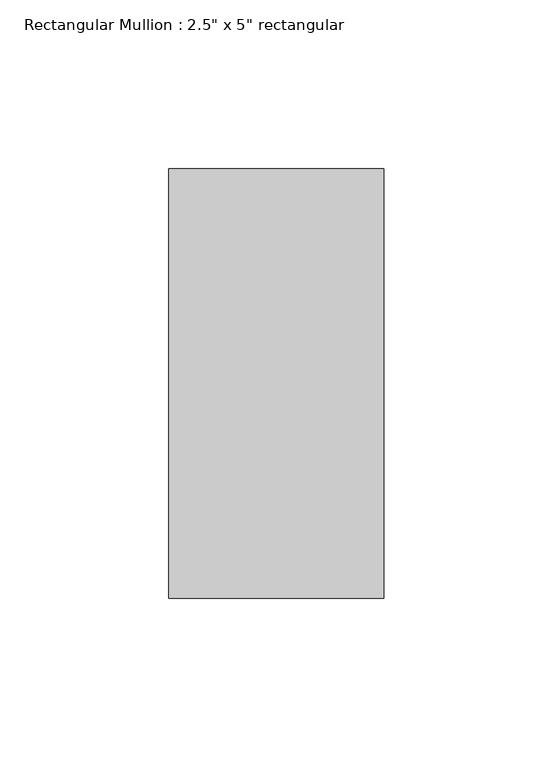
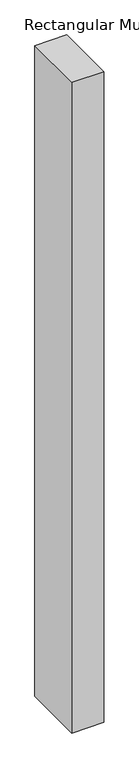
"""IFC4 building model written with IfcOpenShell, lengths in millimetres: member geometry."""

from ifc_helpers import new_model, si_unit, frame, origin, place, context, project, spatial, polyline, outline, extrude, source, transform, mapped, element, save


def member_cd38fec7(model_context):
    return source(origin(), model_context, "Body", "SweptSolid", [
        extrude(outline(polyline([(31.75, 63.5), (31.75, -63.5), (-31.75, -63.5), (-31.75, 63.5), (31.75, 63.5)])), frame((0.0, 0.0, -1366.0685135), z_axis=(0.0, 0.0, 1.0), x_axis=(1.0, 0.0, 0.0)), (0.0, 0.0, 1.0), 1366.0685135),
    ])


if __name__ == "__main__":
    model = new_model("IFC4")
    model_context = context("Model", 3, world=origin())
    ifc_project = project(units=[si_unit("LENGTHUNIT", "METRE", prefix="MILLI")], contexts=[model_context])
    site = spatial("IfcSite", under=ifc_project)
    building = spatial("IfcBuilding", under=site)
    placement = place(None, origin())
    member_shape = member_cd38fec7(model_context)
    element("IfcMember", 1, ObjectType="Rectangular Mullion : 2.5\" x 5\" rectangular", at=placement, inside=building, context=model_context, shape_type="MappedRepresentation", body=[
        mapped(member_shape, transform((0.0, 0.0, 0.0), x_axis=(1.0, 0.0, 0.0), y_axis=(0.0, 1.0, 0.0), z_axis=(0.0, 0.0, 1.0))),
    ])
    save(model, "model.ifc")

# Revit data of these elements
# Type "Rectangular Mullion : 2.5\" x 5\" rectangular"
#   built-in parameter 1007304 = 0.416667 (stored number, unit not read)
#   built-in parameter 1007301 = 0.104167 (stored number, unit not read)
#   built-in parameter 1007300 = 0.104167 (stored number, unit not read)
# Element 1 (IfcMember, "Rectangular Mullion : 2.5\" x 5\" rectangular")
#   Materials on its faces: "Aluminum"
# Materials
#   "Aluminum": class "Metal", colour RGB 247 247 247, transparency 0, Description = "Aluminum 6061", Cost = 0
